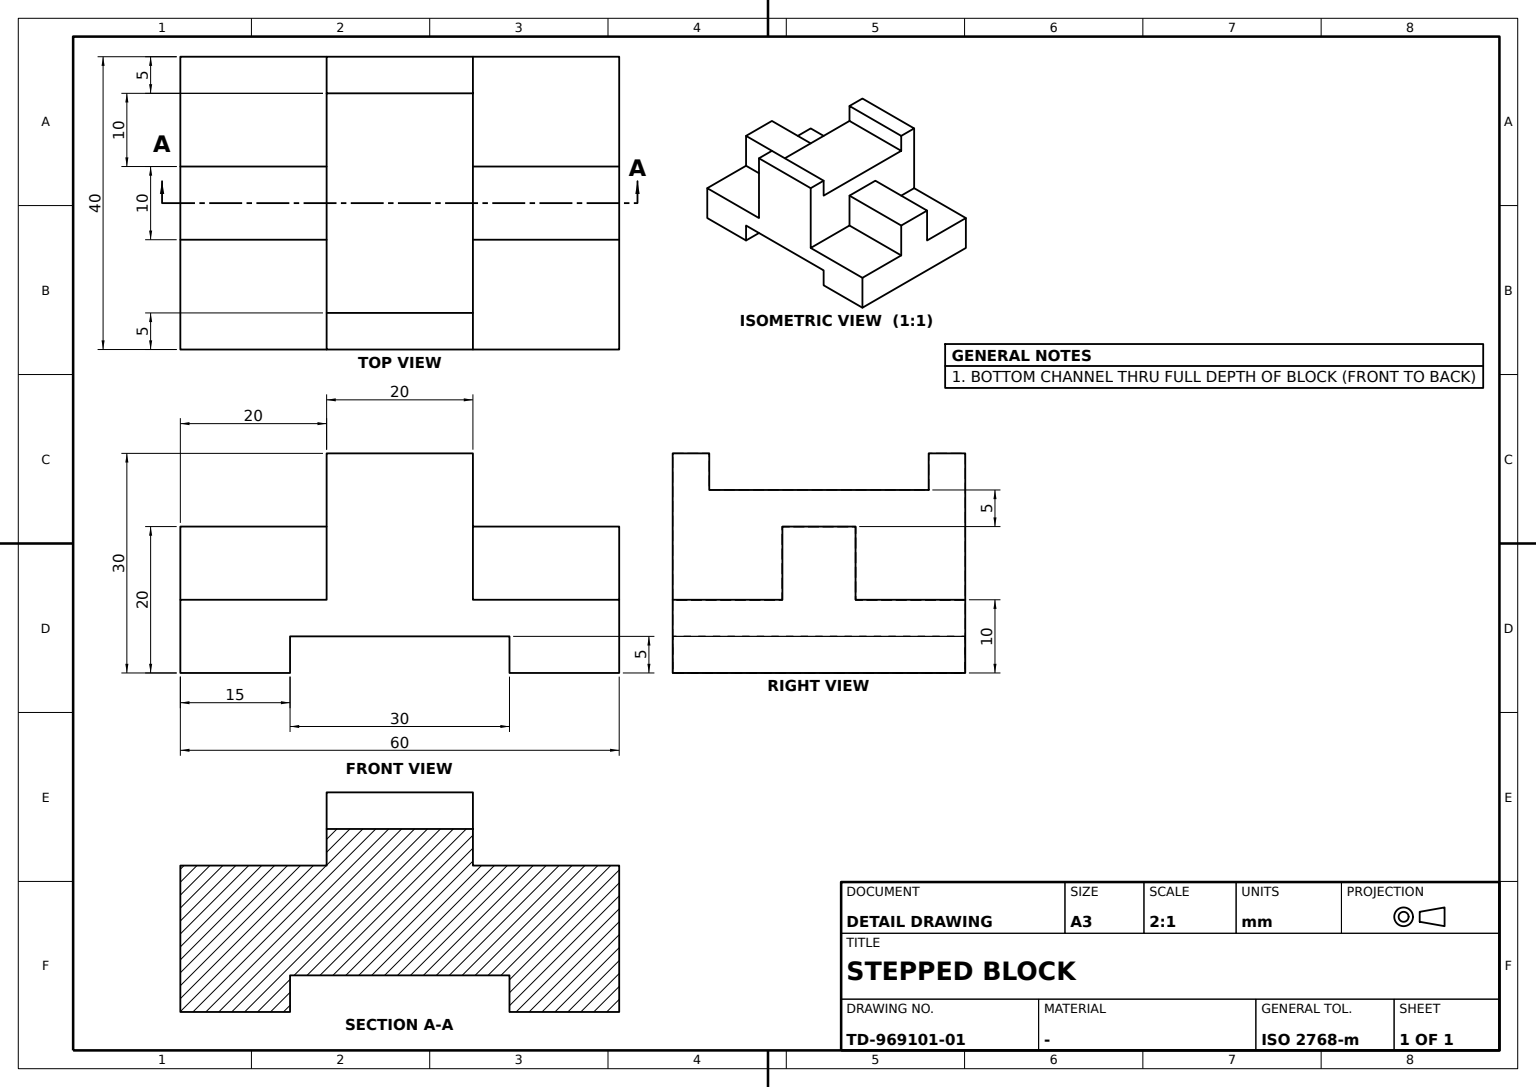
CATIA V5 part; units mm, degrees
sketch "Sketch1" plane through (0, 0, 0) normal (0, 1, 0) x (-1, 0, 0)
  point P0 (-30, 0)
  line L0 (-30, 0) -> (-15, 0)
  line L1 (-15, 0) -> (-15, 5)
  line L2 (-15, 5) -> (15, 5)
  line L3 (15, 5) -> (15, 0)
  point P1 (15, 0)
  line L4 (15, 0) -> (30, 0)
  line L5 (30, 0) -> (30, 10)
  line L6 (30, 10) -> (10, 10)
  line L7 (10, 10) -> (10, 30)
  line L8 (10, 30) -> (-10, 30)
  line L9 (-10, 30) -> (-10, 10)
  point P2 (-10, 10)
  line L10 (-10, 10) -> (-30, 10)
  line L11 (-30, 10) -> (-30, 0)
  dimension "length L2" = 30
  dimension "distance L11 L5" = 60
  dimension "length L8" = 20
  dimension "length L5" = 10
  dimension "distance L8 x axis" = 30
  dimension "distance L2 L6" = 5
  constraint coincidence P0 x-axis
  constraint coincidence P1 x-axis
  constraint coincidence P2 L6
  constraint horizontal L0 x-axis
  constraint horizontal L2 x-axis
  constraint horizontal L4 x-axis
  constraint horizontal L6 x-axis
  constraint horizontal L8 x-axis
  constraint horizontal L10 x-axis
  constraint vertical L1 y-axis
  constraint vertical L3 y-axis
  constraint vertical L5 y-axis
  constraint vertical L7 y-axis
  constraint vertical L9 y-axis
  constraint vertical L11 y-axis
  constraint symmetry L11 L5 y-axis
  constraint symmetry L1 L3 y-axis
  constraint symmetry L9 L7 y-axis
extrude "Pad1" add sketch "Sketch1" against normal blind 40
sketch "Sketch2" plane through (0, 0, 0) normal (1, 0, 0) x (0, 1, 0)
  line L0 (-25, 20) -> (-15, 20)
  line L1 (-15, 20) -> (-15, 10)
  line L2 (-15, 10) -> (-25, 10)
  line L3 (-25, 10) -> (-25, 20)
  line L4 (-40, 30) -> (-40, 10) construction
  line L5 (0, 0) -> (-40, 0) construction
  dimension "length L1" = 10
  dimension "length L0" = 10
  dimension "distance L4 L3" = 15
  dimension "distance L0 L5" = 20
  constraint horizontal L0 x-axis
  constraint horizontal L2 x-axis
  constraint vertical L1 y-axis
  constraint vertical L3 y-axis
extrude "Pad2" add sketch "Sketch2" along normal mid plane 60
sketch "Sketch3" plane through (0, 0, 0) normal (1, 0, 0) x (0, 1, 0)
  line L0 (-35, 30) -> (-5, 30)
  line L1 (-5, 30) -> (-5, 25)
  line L2 (-5, 25) -> (-35, 25)
  line L3 (-35, 25) -> (-35, 30)
  line L4 (-40, 30) -> (-40, 10) construction
  line L5 (0, 30) -> (-40, 30) construction
  dimension "length L3" = 5
  dimension "length L2" = 30
  dimension "distance L3 L4" = 5
  dimension "distance L5 L2" = 5
  constraint horizontal L0 x-axis
  constraint horizontal L2 x-axis
  constraint vertical L1 y-axis
  constraint vertical L3 y-axis
extrude "Pocket1" cut sketch "Sketch3" along normal mid plane 20
properties part number "Stepped mechanical  box"
